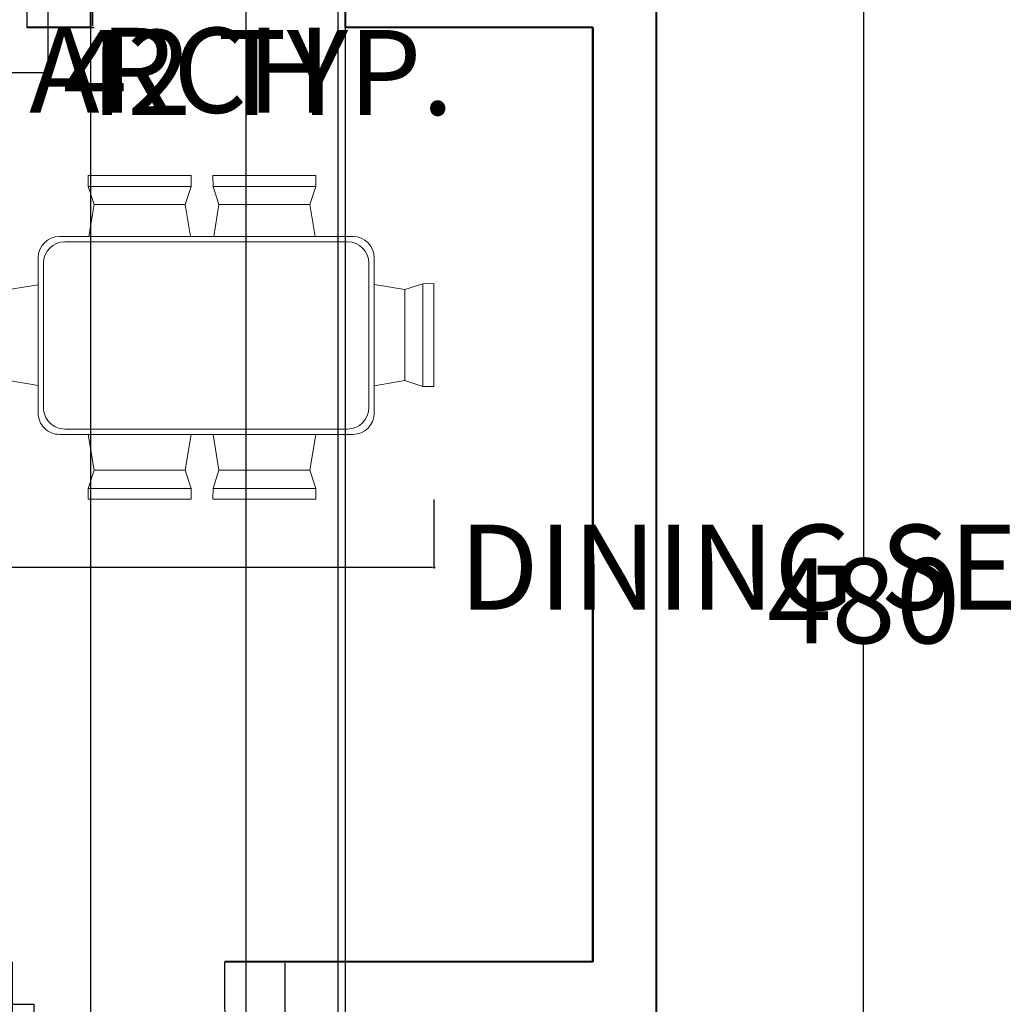
# Model space of a CAD drawing. Units: inches. Extents: x -124 to 612, y -69 to 524.
# Tile 5 of 9: x 148 to 287, y 190 to 329. Entities that reach past the tile are written whole.
import ezdxf
from ezdxf.enums import TextEntityAlignment as Align

# ---------------------------------------------------------------- set-up
doc = ezdxf.new("R2010")
doc.units = ezdxf.units.IN
doc.header["$MEASUREMENT"] = 0
for name, color, linetype, lineweight in [('A-ANNO-DIMS', 2, 'Continuous', 18), ('A-ANNO-TEXT', 1, 'Continuous', 18), ('A-DOOR', 4, 'Continuous', 25), ('A-FURN', 8, 'Continuous', 18), ('A-WALL', 7, 'Continuous', 40)]:
    doc.layers.add(name, color=color, linetype=linetype, lineweight=lineweight)
doc.styles.get("Standard").update_dxf_attribs({"font": 'arial.ttf'})
doc.dimstyles.get("Standard").update_dxf_attribs({"dimtxt": 12, "dimasz": 0.18, "dimexe": 0.18, "dimexo": 0.0625, "dimgap": 0.09, "dimtad": 0, "dimtih": 1, "dimtoh": 1, "dimdec": 0, "dimzin": 0, "dimdsep": 46, "dimlunit": 4, "dimtxsty": 'Standard', "dimcen": 0.09, "dimadec": 0, "dimazin": 0, "dimtfac": 1, "dimtdec": 0, "dimtofl": 0, "dimtmove": 0, "dimatfit": 3, "dimfxl": 1, "dimtolj": 1, "dimtzin": 0, "dimarcsym": 0})

# ---------------------------------------------------------------- blocks, each defined once
blk = doc.blocks.new('A$C6C037A94')
for p, q in [((0.7877, 1.6959), (0.4032, 1.6959)), ((0.4032, 1.6959), (0.4039, 1.6557)), ((0.7877, 1.6557), (0.7877, 1.6959)), ((0.4258, 1.588), (0.4039, 1.6557)), ((0.7877, 1.6557), (0.4039, 1.6557)), ((0.7658, 1.588), (0.7877, 1.6557)), ((0.407, 1.4737), (0.4258, 1.588)), ((0.7658, 1.588), (0.4258, 1.588)), ((0.7847, 1.4737), (0.7658, 1.588)), ((0.307, 1.4737), (0.8868, 1.4737)), ((0.327, 1.4537), (0.8668, 1.4537)), ((0.227, 0.2974), (0.227, 1.3937)), ((0.247, 0.3174), (0.247, 1.3737)), ((0.9468, 1.3737), (0.9468, 0.3174)), ((0.9668, 1.3937), (0.9668, 0.2974)), ((0, 1.2552), (0, 0.8707)), ((0.0402, 1.2552), (0, 1.2552)), ((0.0402, 1.2552), (0.0402, 0.8714)), ((0.1079, 1.2333), (0.0402, 1.2552)), ((0.227, 1.2529), (0.1079, 1.2333)), ((0.9668, 1.2553), (1.1005, 1.2333)), ((1.1005, 1.2333), (1.1682, 1.2552)), ((1.1682, 1.2552), (1.2084, 1.2552)), ((1.1682, 1.2552), (1.1682, 0.8714)), ((1.2084, 1.2552), (1.2084, 0.8707)), ((0.1079, 1.2333), (0.1079, 0.8933)), ((1.1005, 1.2333), (1.1005, 0.8933)), ((0.1079, 0.8933), (0.0402, 0.8714)), ((0.227, 0.8736), (0.1079, 0.8933)), ((0.9668, 0.8712), (1.1005, 0.8933)), ((1.1005, 0.8933), (1.1682, 0.8714)), ((0, 0.8707), (0.0402, 0.8714)), ((1.2084, 0.8707), (1.1682, 0.8714)), ((0, 0.7888), (0, 0.4043)), ((0.0402, 0.7888), (0, 0.7888)), ((0.0402, 0.7888), (0.0402, 0.405)), ((0.1079, 0.7669), (0.0402, 0.7888)), ((0.227, 0.7865), (0.1079, 0.7669)), ((0.9668, 0.7889), (1.1005, 0.7669)), ((1.1005, 0.7669), (1.1682, 0.7888)), ((1.1682, 0.7888), (1.1682, 0.405)), ((1.1682, 0.7888), (1.2084, 0.7888)), ((1.2084, 0.7888), (1.2084, 0.4043)), ((0.1079, 0.7669), (0.1079, 0.4269)), ((1.1005, 0.7669), (1.1005, 0.4269)), ((0, 0.4043), (0.0402, 0.405)), ((0.1079, 0.4269), (0.0402, 0.405)), ((0.227, 0.4072), (0.1079, 0.4269)), ((0.9668, 0.4048), (1.1005, 0.4269)), ((1.1005, 0.4269), (1.1682, 0.405)), ((1.2084, 0.4043), (1.1682, 0.405)), ((0.8668, 0.2374), (0.327, 0.2374)), ((0.8868, 0.2174), (0.307, 0.2174)), ((0.4078, 0.2174), (0.4258, 0.1079)), ((0.7839, 0.2174), (0.7658, 0.1079)), ((0.4258, 0.1079), (0.4039, 0.0402)), ((0.7658, 0.1079), (0.4258, 0.1079)), ((0.7658, 0.1079), (0.7877, 0.0402)), ((0.4032, 0), (0.4039, 0.0402)), ((0.7877, 0.0402), (0.4039, 0.0402)), ((0.7877, 0.0402), (0.7877, 0)), ((0.7877, 0), (0.4032, 0))]:
    blk.add_line(p, q)
for centre, start, end in [((0.307, 1.3937), 90, 180), ((0.8868, 1.3937), 360, 90), ((0.327, 1.3737), 90, 180), ((0.8668, 1.3737), 360, 90), ((0.307, 0.2974), 180, 270), ((0.327, 0.3174), 180, 270), ((0.8668, 0.3174), 270, 0), ((0.8868, 0.2974), 270, 360)]:
    blk.add_arc(centre, 0.08, start, end)
blk = doc.blocks.new('DOOR-36IN-SINGLE')
for p, q in [((0, 6), (0, 0)), ((3, 6), (3, 0)), ((39, 6), (39, 0)), ((42, 6), (42, 0))]:
    blk.add_line(p, q)
blk.add_lwpolyline([(39, 6), (36, 6), (36, 42), (39, 42)], close=True)
blk.add_arc((37.5, 7.5), 34.53, 87.5104, 182.4896)
blk = doc.blocks.new('DOOR-30IN-STAIR')
for p, q in [((0, 30.04), (0, 36.04)), ((3, 30.04), (3, 36.04)), ((33, 30.04), (33, 36.04)), ((36, 30.04), (36, 36.04))]:
    blk.add_line(p, q)
blk.add_lwpolyline([(3, 30.04), (6, 30.04), (6, 0.04), (3, 0.04)], close=True)
blk.add_arc((4.5, 28.54), 28.54, 266.9872, 3.0128)
blk = doc.blocks.new('*D23')
at = {"layer": 'A-ANNO-DIMS', "color": 0, "lineweight": -2, "transparency": 16777216}
for p, q in [((152.41, 370.45), (158.89, 370.45)), ((158.71, 370.27), (158.71, 355.54)), ((158.71, 328.21), (158.71, 342.94)), ((152.41, 328.03), (158.89, 328.03))]:
    blk.add_line(p, q, dxfattribs=at)
at = {"layer": 'A-ANNO-DIMS', "color": 0, "transparency": 16777216}
for points in [[(158.68, 370.27), (158.74, 370.27), (158.71, 370.45)], [(158.68, 328.21), (158.74, 328.21), (158.71, 328.03)]]:
    blk.add_solid(points, dxfattribs=at)
at = {"layer": 'Defpoints', "color": 0, "transparency": 16777216}
for p in [(152.35, 370.45), (158.71, 370.45), (152.35, 328.03)]:
    blk.add_point(p, dxfattribs=at)
at = {"layer": 'A-ANNO-DIMS', "color": 0, "transparency": 16777216, "insert": (158.71, 349.24), "char_height": 12, "attachment_point": 5}
blk.add_mtext('\\A1;BEDROOM DOOR 42 TYP.', dxfattribs=at)
blk = doc.blocks.new('*D24')
at = {"layer": 'A-ANNO-DIMS', "color": 0, "lineweight": -2, "transparency": 16777216}
for p, q in [((110.35, 327.97), (110.35, 321.49)), ((152.35, 327.97), (152.35, 321.49)), ((110.53, 321.67), (152.17, 321.67)), ((152.35, 321.67), (152.53, 321.67))]:
    blk.add_line(p, q, dxfattribs=at)
at = {"layer": 'A-ANNO-DIMS', "color": 0, "transparency": 16777216}
for points in [[(110.53, 321.7), (110.53, 321.64), (110.35, 321.67)], [(152.17, 321.7), (152.17, 321.64), (152.35, 321.67)]]:
    blk.add_solid(points, dxfattribs=at)
at = {"layer": 'Defpoints', "color": 0, "transparency": 16777216}
for p in [(110.35, 328.03), (152.35, 328.03), (152.35, 321.67)]:
    blk.add_point(p, dxfattribs=at)
at = {"layer": 'A-ANNO-DIMS', "color": 0, "transparency": 16777216, "insert": (182.07, 321.67), "char_height": 12, "attachment_point": 5}
blk.add_mtext('\\A1;42 TYP.', dxfattribs=at)
blk = doc.blocks.new('*D32')
at = {"layer": 'A-ANNO-DIMS', "color": 0, "lineweight": -2, "transparency": 16777216}
for p, q in [((208.66, 346.55), (208.66, 343.03)), ((226.48, 346.55), (226.48, 343.03)), ((208.66, 343.21), (208.48, 343.21)), ((226.3, 343.21), (208.84, 343.21))]:
    blk.add_line(p, q, dxfattribs=at)
at = {"layer": 'A-ANNO-DIMS', "color": 0, "transparency": 16777216}
for points in [[(208.84, 343.24), (208.84, 343.18), (208.66, 343.21)], [(226.3, 343.24), (226.3, 343.18), (226.48, 343.21)]]:
    blk.add_solid(points, dxfattribs=at)
at = {"layer": 'Defpoints', "color": 0, "transparency": 16777216}
for p in [(208.66, 346.62), (226.48, 346.62), (208.66, 343.21)]:
    blk.add_point(p, dxfattribs=at)
at = {"layer": 'A-ANNO-DIMS', "color": 0, "transparency": 16777216, "insert": (179.75, 343.21), "char_height": 12, "attachment_point": 5}
blk.add_mtext('\\A1;18 TYP.', dxfattribs=at)
blk = doc.blocks.new('*D39')
at = {"layer": 'A-ANNO-DIMS', "color": 0, "lineweight": -2, "transparency": 16777216}
for p, q in [((180.41, 196.03), (186, 196.03)), ((185.82, 195.85), (185.82, 184.12)), ((185.82, 159.78), (185.82, 171.51)), ((180.41, 159.6), (186, 159.6))]:
    blk.add_line(p, q, dxfattribs=at)
at = {"layer": 'A-ANNO-DIMS', "color": 0, "transparency": 16777216}
for points in [[(185.79, 195.85), (185.85, 195.85), (185.82, 196.03)], [(185.79, 159.78), (185.85, 159.78), (185.82, 159.6)]]:
    blk.add_solid(points, dxfattribs=at)
at = {"layer": 'Defpoints', "color": 0, "transparency": 16777216}
for p in [(180.35, 196.03), (185.82, 196.03), (180.35, 159.6)]:
    blk.add_point(p, dxfattribs=at)
at = {"layer": 'A-ANNO-DIMS', "color": 0, "transparency": 16777216, "insert": (185.82, 177.82), "char_height": 12, "attachment_point": 5}
blk.add_mtext('\\A1;STAIR DOOR 36 TYP.', dxfattribs=at)
blk = doc.blocks.new('*D45')
at = {"layer": 'A-ANNO-DIMS', "color": 0, "lineweight": -2, "transparency": 16777216}
for p, q in [((142.74, 261.33), (142.74, 251.59)), ((206.86, 261.33), (206.86, 251.59)), ((142.92, 251.77), (206.68, 251.77)), ((206.86, 251.77), (207.04, 251.77))]:
    blk.add_line(p, q, dxfattribs=at)
at = {"layer": 'A-ANNO-DIMS', "color": 0, "transparency": 16777216}
for points in [[(142.92, 251.8), (142.92, 251.74), (142.74, 251.77)], [(206.68, 251.8), (206.68, 251.74), (206.86, 251.77)]]:
    blk.add_solid(points, dxfattribs=at)
at = {"layer": 'Defpoints', "color": 0, "transparency": 16777216}
for p in [(142.74, 261.39), (206.86, 261.39), (206.86, 251.77)]:
    blk.add_point(p, dxfattribs=at)
at = {"layer": 'A-ANNO-DIMS', "color": 0, "transparency": 16777216, "insert": (265.7, 251.77), "char_height": 12, "attachment_point": 5}
blk.add_mtext('\\A1;DINING SET 64', dxfattribs=at)
blk = doc.blocks.new('*D48')
at = {"layer": 'A-ANNO-DIMS', "color": 0, "lineweight": -2, "transparency": 16777216}
for p, q in [((238.41, 487.03), (267.78, 487.03)), ((267.6, 486.85), (267.6, 253.25)), ((267.6, 7.21), (267.6, 240.81)), ((238.41, 7.03), (267.78, 7.03))]:
    blk.add_line(p, q, dxfattribs=at)
at = {"layer": 'A-ANNO-DIMS', "color": 0, "transparency": 16777216}
for points in [[(267.57, 486.85), (267.63, 486.85), (267.6, 487.03)], [(267.57, 7.21), (267.63, 7.21), (267.6, 7.03)]]:
    blk.add_solid(points, dxfattribs=at)
at = {"layer": 'Defpoints', "color": 0, "transparency": 16777216}
for p in [(238.35, 487.03), (267.6, 487.03), (238.35, 7.03)]:
    blk.add_point(p, dxfattribs=at)
at = {"layer": 'A-ANNO-DIMS', "color": 0, "transparency": 16777216, "insert": (267.6, 247.03), "char_height": 12, "attachment_point": 5}
blk.add_mtext('\\A1;480', dxfattribs=at)
blk = doc.blocks.new('*D52')
at = {"layer": 'A-ANNO-DIMS', "color": 0, "lineweight": -2, "transparency": 16777216}
for p, q in [((158.35, 327.97), (158.35, -22.4)), ((194.35, 327.97), (194.35, -22.4)), ((158.53, -22.22), (167.67, -22.22)), ((194.17, -22.22), (185.03, -22.22))]:
    blk.add_line(p, q, dxfattribs=at)
at = {"layer": 'A-ANNO-DIMS', "color": 0, "transparency": 16777216}
for points in [[(158.53, -22.19), (158.53, -22.25), (158.35, -22.22)], [(194.17, -22.19), (194.17, -22.25), (194.35, -22.22)]]:
    blk.add_solid(points, dxfattribs=at)
at = {"layer": 'Defpoints', "color": 0, "transparency": 16777216}
for p in [(158.35, 328.03), (194.35, 328.03), (194.35, -22.22)]:
    blk.add_point(p, dxfattribs=at)
at = {"layer": 'A-ANNO-DIMS', "color": 0, "transparency": 16777216, "insert": (176.35, -22.22), "char_height": 12, "attachment_point": 5}
blk.add_mtext('\\A1;36', dxfattribs=at)
blk = doc.blocks.new('*D65')
at = {"layer": 'A-ANNO-DIMS', "color": 0, "lineweight": -2, "transparency": 16777216}
for p, q in [((180.35, 112.09), (180.35, 516.46)), ((180.53, 516.28), (193.17, 516.28)), ((193.35, 112.09), (193.35, 516.46)), ((193.35, 516.28), (193.53, 516.28))]:
    blk.add_line(p, q, dxfattribs=at)
at = {"layer": 'A-ANNO-DIMS', "color": 0, "transparency": 16777216}
for points in [[(180.53, 516.31), (180.53, 516.25), (180.35, 516.28)], [(193.17, 516.31), (193.17, 516.25), (193.35, 516.28)]]:
    blk.add_solid(points, dxfattribs=at)
at = {"layer": 'Defpoints', "color": 0, "transparency": 16777216}
for p in [(193.35, 516.28), (180.35, 112.03), (193.35, 112.03)]:
    blk.add_point(p, dxfattribs=at)
at = {"layer": 'A-ANNO-DIMS', "color": 0, "transparency": 16777216, "insert": (201.65, 516.28), "char_height": 12, "attachment_point": 5}
blk.add_mtext('\\A1;13', dxfattribs=at)

msp = doc.modelspace()

# ---------------------------------------------------------------- linework, layer by layer
at = {"layer": 'A-WALL'}
for p, q in [((158.3513, 334.0291), (158.3513, 328.0291)), ((194.3513, 334.0291), (194.3513, 328.0291)), ((158.3513, 328.0291), (149.3513, 328.0291)), ((229.3513, 328.0291), (194.3513, 328.0291)), ((229.3513, 328.0291), (229.3513, 196.0291)), ((229.3513, 196.0291), (229.3513, 328.0291)), ((229.3513, 196.0291), (177.3513, 196.0291))]:
    msp.add_line(p, q, dxfattribs=at)
msp.add_lwpolyline([(10.3513, 7.0291), (238.3513, 7.0291), (238.3513, 487.0291), (10.3513, 487.0291)], close=True, dxfattribs=at)

# ---------------------------------------------------------------- block references
at = {"layer": 'A-DOOR'}
for name, p in [('DOOR-36IN-SINGLE', (110.351, 328.029)), ('DOOR-30IN-STAIR', (144.351, 159.99))]:
    msp.add_blockref(name, p, dxfattribs=at)
at = {"layer": 'A-FURN', "xscale": 37.81157970897361, "yscale": 37.81157970897361, "zscale": 37.81157970897361, "rotation": 270}
msp.add_blockref('A$C6C037A94', (142.7351, 307.0846), dxfattribs=at)

# ---------------------------------------------------------------- texts
at = {"layer": 'A-ANNO-TEXT'}
msp.add_text('ARCH', height=12, dxfattribs=at).set_placement((171.042, 315.9647), align=Align.CENTER)

# ---------------------------------------------------------------- dimensions: what is measured, and where the dimension line sits
at = {"layer": 'A-ANNO-DIMS'}
for base, p1, p2, picture, middle in [((193.3513, 516.2791), (180.3513, 112.0291), (193.3513, 112.0291), '*D65', (201.6513, 516.2791)), ((194.3513, -22.2209), (158.3513, 328.0291), (194.3513, 328.0291), '*D52', (176.3513, -22.2209))]:
    dim = msp.add_linear_dim(base=base, p1=p1, p2=p2, dimstyle='Standard', override={"dimdec": 0, "dimlfac": 1, "dimrnd": 0, "dimzin": 0, "dimdsep": 46, "dimlunit": 2}, dxfattribs=at)
    dim.commit()
    dim.dimension.update_dxf_attribs({"geometry": picture, "text_midpoint": middle})
dim = msp.add_linear_dim(base=(267.6013, 487.0291), p1=(238.3513, 7.0291), p2=(238.3513, 487.0291), angle=90, dimstyle='Standard', override={"dimdec": 0, "dimlfac": 1, "dimrnd": 0, "dimzin": 0, "dimdsep": 46, "dimlunit": 2}, dxfattribs=at)
dim.commit()
dim.dimension.update_dxf_attribs({"geometry": '*D48', "text_midpoint": (267.6013, 247.0291)})
for base, p1, p2, angle, text, picture, middle in [((158.7144, 370.4495), (152.3513, 328.0291), (152.3513, 370.4495), 90, 'BEDROOM DOOR <> TYP.', '*D23', (158.7144, 349.2393)), ((208.6637, 343.2121), (226.4757, 346.6153), (208.6637, 346.6153), 180, '<> TYP.', '*D32', (179.7525, 343.2121)), ((185.8151, 196.0291), (180.3513, 159.6038), (180.3513, 196.0291), 90, 'STAIR DOOR <> TYP.', '*D39', (185.8151, 177.8164))]:
    dim = msp.add_linear_dim(base=base, p1=p1, p2=p2, angle=angle, text=text, dimstyle='Standard', override={"dimdec": 0, "dimlfac": 1, "dimrnd": 0, "dimzin": 0, "dimdsep": 46, "dimlunit": 2}, dxfattribs=at)
    dim.commit()
    dim.dimension.update_dxf_attribs({"geometry": picture, "text_midpoint": middle})
for base, p1, p2, text, picture, middle in [((152.3513, 321.666), (110.3513, 328.0291), (152.3513, 328.0291), '<> TYP.', '*D24', (182.0688, 321.666)), ((206.8595, 251.775), (142.7351, 261.3936), (206.8595, 261.3936), 'DINING SET <>', '*D45', (265.697, 251.775))]:
    dim = msp.add_linear_dim(base=base, p1=p1, p2=p2, text=text, dimstyle='Standard', override={"dimdec": 0, "dimlfac": 1, "dimrnd": 0, "dimzin": 0, "dimdsep": 46, "dimlunit": 2}, dxfattribs=at)
    dim.commit()
    dim.dimension.update_dxf_attribs({"geometry": picture, "text_midpoint": middle})

doc.saveas('drawing.dxf')
